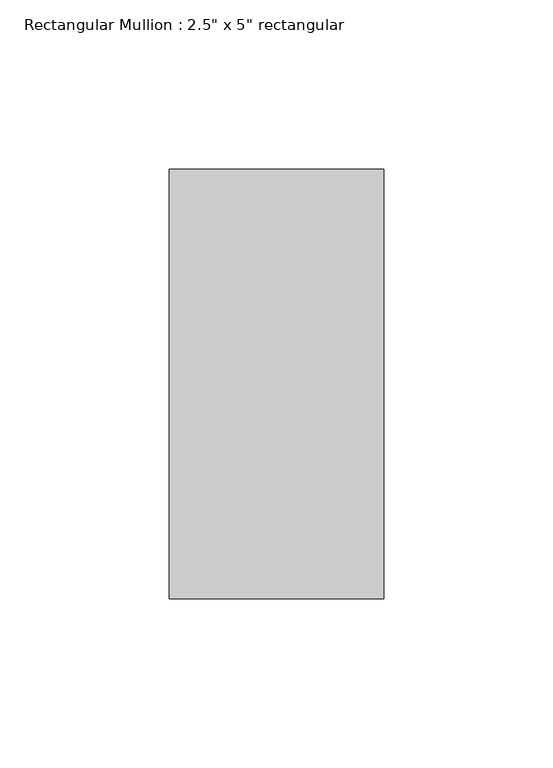
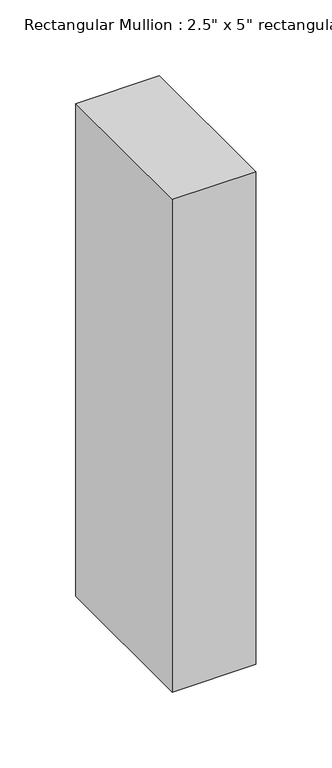
"""IFC4 building model written with IfcOpenShell, lengths in millimetres: member geometry."""

from ifc_helpers import new_model, si_unit, frame, origin, place, context, project, spatial, polyline, outline, extrude, source, transform, mapped, element, save


def member_467e6651(model_context):
    return source(origin(), model_context, "Body", "SweptSolid", [
        extrude(outline(polyline([(31.75, 63.5), (31.75, -63.5), (-31.75, -63.5), (-31.75, 63.5), (31.75, 63.5)])), frame((0.0, 0.0, -396.24), z_axis=(0.0, 0.0, 1.0), x_axis=(1.0, 0.0, 0.0)), (0.0, 0.0, 1.0), 396.24),
    ])


if __name__ == "__main__":
    model = new_model("IFC4")
    model_context = context("Model", 3, world=origin())
    ifc_project = project(units=[si_unit("LENGTHUNIT", "METRE", prefix="MILLI")], contexts=[model_context])
    site = spatial("IfcSite", under=ifc_project)
    building = spatial("IfcBuilding", under=site)
    placement = place(None, origin())
    member_shape = member_467e6651(model_context)
    element("IfcMember", 1, ObjectType="Rectangular Mullion : 2.5\" x 5\" rectangular", at=placement, inside=building, context=model_context, shape_type="MappedRepresentation", body=[
        mapped(member_shape, transform((0.0, 0.0, 0.0), x_axis=(1.0, 0.0, 0.0), y_axis=(0.0, 1.0, 0.0), z_axis=(0.0, 0.0, 1.0))),
    ])
    save(model, "model.ifc")

# Revit data of these elements
# Type "Rectangular Mullion : 2.5\" x 5\" rectangular"
#   built-in parameter 1007304 = 0.416667 (stored number, unit not read)
#   built-in parameter 1007301 = 0.104167 (stored number, unit not read)
#   built-in parameter 1007300 = 0.104167 (stored number, unit not read)
# Element 1 (IfcMember, "Rectangular Mullion : 2.5\" x 5\" rectangular")
#   Materials on its faces: "Aluminum"
# Materials
#   "Aluminum": class "Metal", colour RGB 247 247 247, transparency 0, Description = "Aluminum 6061", Cost = 0
